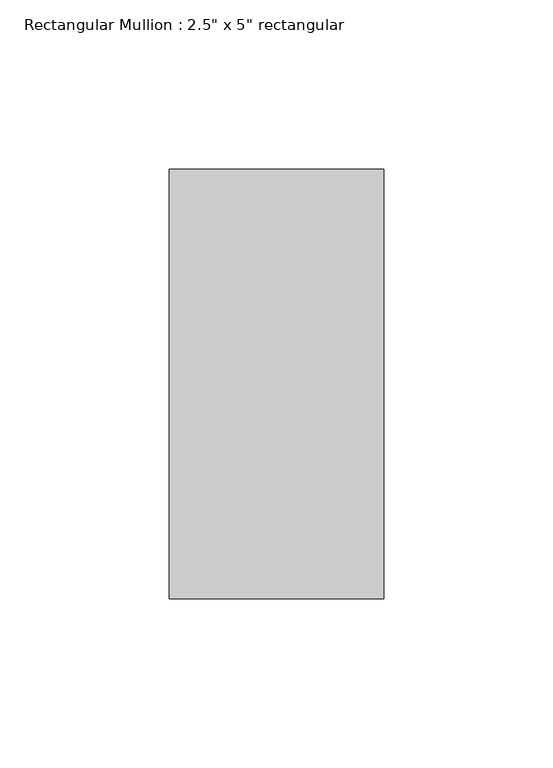
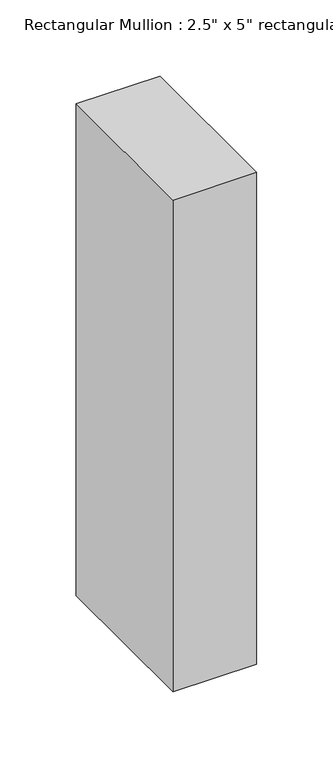
"""IFC4 building model written with IfcOpenShell, lengths in millimetres: member geometry."""

from ifc_helpers import new_model, si_unit, frame, origin, place, context, project, spatial, polyline, outline, extrude, source, transform, mapped, element, save


def member_951753a7(model_context):
    return source(origin(), model_context, "Body", "SweptSolid", [
        extrude(outline(polyline([(31.75, 63.5), (31.75, -63.5), (-31.75, -63.5), (-31.75, 63.5), (31.75, 63.5)])), frame((0.0, 0.0, -393.7), z_axis=(0.0, 0.0, 1.0), x_axis=(1.0, 0.0, 0.0)), (0.0, 0.0, 1.0), 393.7),
    ])


if __name__ == "__main__":
    model = new_model("IFC4")
    model_context = context("Model", 3, world=origin())
    ifc_project = project(units=[si_unit("LENGTHUNIT", "METRE", prefix="MILLI")], contexts=[model_context])
    site = spatial("IfcSite", under=ifc_project)
    building = spatial("IfcBuilding", under=site)
    placement = place(None, origin())
    member_shape = member_951753a7(model_context)
    element("IfcMember", 1, ObjectType="Rectangular Mullion : 2.5\" x 5\" rectangular", at=placement, inside=building, context=model_context, shape_type="MappedRepresentation", body=[
        mapped(member_shape, transform((0.0, 0.0, 0.0), x_axis=(1.0, 0.0, 0.0), y_axis=(0.0, 1.0, 0.0), z_axis=(0.0, 0.0, 1.0))),
    ])
    save(model, "model.ifc")

# Revit data of these elements
# Type "Rectangular Mullion : 2.5\" x 5\" rectangular"
#   built-in parameter 1007304 = 0.416667 (stored number, unit not read)
#   built-in parameter 1007301 = 0.104167 (stored number, unit not read)
#   built-in parameter 1007300 = 0.104167 (stored number, unit not read)
# Element 1 (IfcMember, "Rectangular Mullion : 2.5\" x 5\" rectangular")
#   Materials on its faces: "Aluminum"
# Materials
#   "Aluminum": class "Metal", colour RGB 247 247 247, transparency 0, Description = "Aluminum 6061", Cost = 0
